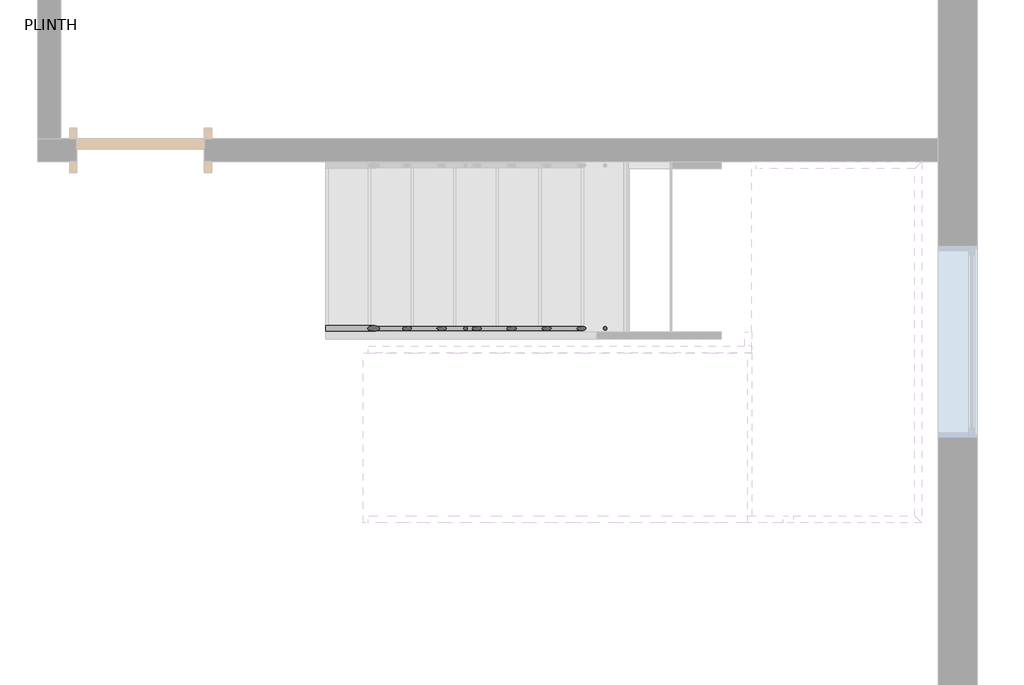
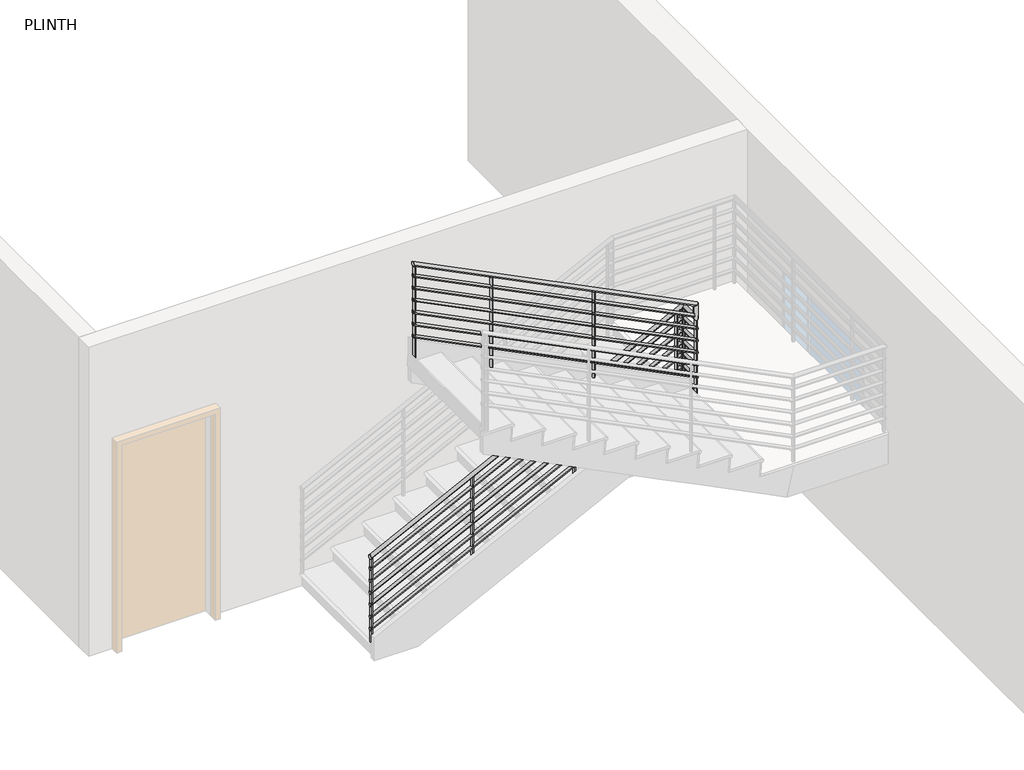
# One storey, part 2 of 4: 1 railing.
"""IFC4 building model written with IfcOpenShell, lengths in millimetres."""

from ifc_helpers import new_model, si_unit, point, frame, frame_2d, origin, place, context, project, spatial, circle_curve, ellipse_curve, trimmed, segment, composite_curve, outline, extrude, element, save
from ifc_brep_helpers import plane_surface, cylinder_surface, advanced_brep

model = new_model("IFC4")

# Units and contexts
model_context = context("Model", 3, world=origin())
ifc_project = project(units=[si_unit("LENGTHUNIT", "METRE", prefix="MILLI")], contexts=[model_context])

# Site, building, storey
site = spatial("IfcSite", under=ifc_project)
building = spatial("IfcBuilding", under=site)
storey = spatial("IfcBuildingStorey", under=building, Name="PLINTH", Elevation=0.0)

# Railing
placement = place(None, origin())
element("IfcRailing", 1, ObjectType="900mm Pipe", at=placement, inside=storey, context=model_context, shape_type="SolidModel", body=[
    advanced_brep(
    [(6849.4583908, 2412.6640673, 1030.0393202), (6849.4583908, 2452.6640673, 1030.0393202), (9913.9141188, 2412.6640673, 2562.2671843), (9949.6912065, 2452.6640673, 2580.1557281)],
    [
        (0, 1, ellipse_curve(frame((6849.4583908, 2432.6640673, 1030.0393202), z_axis=(-1.0, 0.0, 0.0), x_axis=(0.0, 0.0, -1.0)), 22.3606798, 20.0)),
        (1, 0, ellipse_curve(frame((6849.4583908, 2432.6640673, 1030.0393202), z_axis=(-1.0, 0.0, 0.0), x_axis=(0.0, 0.0, -1.0)), 22.3606798, 20.0)),
        (2, 3, ellipse_curve(frame((9931.8026627, 2432.6640673, 2571.2114562), z_axis=(0.632455532033675, -0.7071067811865486, 0.3162277660168374), x_axis=(-0.6324555320336768, -0.7071067811865465, -0.3162277660168383)), 28.2842712, 20.0)),
        (3, 2, ellipse_curve(frame((9931.8026627, 2432.6640673, 2571.2114562), z_axis=(0.632455532033675, -0.7071067811865486, 0.3162277660168374), x_axis=(-0.6324555320336768, -0.7071067811865465, -0.3162277660168383)), 28.2842712, 20.0)),
        (0, 2),
        (3, 1),
    ],
    [
        plane_surface(frame((6849.4583908, 2432.6640673, 1052.4), z_axis=(-1.0, 0.0, 0.0), x_axis=(0.0, 1.0, 0.0))),
        plane_surface(frame((9922.8583908, 2432.6640673, 2589.1), z_axis=(0.6324555320336751, -0.7071067811865487, 0.31622776601683744), x_axis=(0.7745966692414842, 0.5773502691896254, -0.25819888974716015))),
        cylinder_surface(frame((6858.4026627, 2432.6640673, 1034.5114562), z_axis=(-0.894427190999916, 0.0, -0.4472135954999578), x_axis=(0.0, 1.0, 0.0)), 20.0),
    ],
    [
        (0, [[1, 2]]),
        (1, [[3, 4]]),
        (2, [[-1, 5, -4, 6]]),
        (2, [[-2, -6, -3, -5]]),
    ],
),
    advanced_brep(
    [(9902.8583908, 2405.8312516, 2556.4), (9942.8583908, 2441.6083392, 2556.4), (9902.8583908, 2231.8640673, 2556.4), (9942.8583908, 2231.8640673, 2556.4)],
    [
        (0, 1, ellipse_curve(frame((9922.8583908, 2423.7197954, 2556.4), z_axis=(-0.632455532033675, 0.7071067811865486, -0.3162277660168374), x_axis=(0.6324555320336768, 0.7071067811865465, 0.3162277660168383)), 28.2842712, 20.0)),
        (1, 0, ellipse_curve(frame((9922.8583908, 2423.7197954, 2556.4), z_axis=(-0.632455532033675, 0.7071067811865486, -0.3162277660168374), x_axis=(0.6324555320336768, 0.7071067811865465, 0.3162277660168383)), 28.2842712, 20.0)),
        (2, 3, ellipse_curve(frame((9922.8583908, 2231.8640673, 2556.4), z_axis=(0.0, -0.7071067811865476, 0.7071067811865476), x_axis=(0.0, 0.7071067811865474, 0.7071067811865476)), 28.2842712, 20.0)),
        (3, 2, ellipse_curve(frame((9922.8583908, 2231.8640673, 2556.4), z_axis=(0.0, -0.7071067811865476, 0.7071067811865476), x_axis=(0.0, 0.7071067811865474, 0.7071067811865476)), 28.2842712, 20.0)),
        (0, 2),
        (3, 1),
    ],
    [
        plane_surface(frame((9922.8583908, 2432.6640673, 2576.4), z_axis=(-0.6324555320336751, 0.7071067811865487, -0.31622776601683744), x_axis=(0.7745966692414842, 0.5773502691896254, -0.25819888974716015))),
        plane_surface(frame((9922.8583908, 2251.8640673, 2576.4), z_axis=(0.0, -0.7071067811865476, 0.7071067811865476), x_axis=(1.0, 0.0, 0.0))),
        cylinder_surface(frame((9922.8583908, 2432.6640673, 2556.4), z_axis=(0.0, 1.0, 0.0), x_axis=(1.0, 0.0, 0.0)), 20.0),
    ],
    [
        (0, [[1, 2]]),
        (1, [[3, 4]]),
        (2, [[-1, 5, -4, 6]]),
        (2, [[-2, -6, -3, -5]]),
    ],
),
    advanced_brep(
    [(9902.8583908, 2231.8640673, 2556.4), (9942.8583908, 2231.8640673, 2556.4), (9902.8583908, 2231.8640673, 2681.3786405), (9942.8583908, 2231.8640673, 2706.1)],
    [
        (0, 1, ellipse_curve(frame((9922.8583908, 2231.8640673, 2556.4), z_axis=(0.0, 0.7071067811865476, -0.7071067811865476), x_axis=(0.0, -0.7071067811865476, -0.7071067811865474)), 28.2842712, 20.0)),
        (1, 0, ellipse_curve(frame((9922.8583908, 2231.8640673, 2556.4), z_axis=(0.0, 0.7071067811865476, -0.7071067811865476), x_axis=(0.0, -0.7071067811865476, -0.7071067811865474)), 28.2842712, 20.0)),
        (2, 3, ellipse_curve(frame((9922.8583908, 2231.8640673, 2693.7393202), z_axis=(-0.5257311121191335, 0.0, 0.8506508083520401), x_axis=(-0.8506508083520401, 0.0, -0.5257311121191331)), 23.5114101, 20.0)),
        (3, 2, ellipse_curve(frame((9922.8583908, 2231.8640673, 2693.7393202), z_axis=(-0.5257311121191335, 0.0, 0.8506508083520401), x_axis=(-0.8506508083520401, 0.0, -0.5257311121191331)), 23.5114101, 20.0)),
        (0, 2),
        (3, 1),
    ],
    [
        plane_surface(frame((9922.8583908, 2231.8640673, 2556.4), z_axis=(0.0, 0.7071067811865476, -0.7071067811865476), x_axis=(1.0, 0.0, 0.0))),
        plane_surface(frame((9922.8583908, 2231.8640673, 2693.7393202), z_axis=(-0.5257311121191335, 0.0, 0.8506508083520401), x_axis=(0.8506508083520401, 0.0, 0.5257311121191335))),
        cylinder_surface(frame((9922.8583908, 2231.8640673, 2556.4), z_axis=(0.0, 0.0, -1.0), x_axis=(1.0, 0.0, 0.0)), 20.0),
    ],
    [
        (0, [[1, 2]]),
        (1, [[3, 4]]),
        (2, [[-1, 5, -4, 6]]),
        (2, [[-2, -6, -3, -5]]),
    ],
),
    advanced_brep(
    [(9922.8583908, 2251.8640673, 2693.7393202), (9922.8583908, 2211.8640673, 2693.7393202), (7154.2583908, 2251.8640673, 4078.0393202), (7154.2583908, 2211.8640673, 4078.0393202)],
    [
        (0, 1, ellipse_curve(frame((9922.8583908, 2231.8640673, 2693.7393202), z_axis=(0.5257311121191335, 0.0, -0.8506508083520401), x_axis=(0.8506508083520399, 0.0, 0.5257311121191337)), 23.5114101, 20.0)),
        (1, 0, ellipse_curve(frame((9922.8583908, 2231.8640673, 2693.7393202), z_axis=(0.5257311121191335, 0.0, -0.8506508083520401), x_axis=(0.8506508083520399, 0.0, 0.5257311121191337)), 23.5114101, 20.0)),
        (2, 3, ellipse_curve(frame((7154.2583908, 2231.8640673, 4078.0393202), z_axis=(-1.0, 0.0, 0.0), x_axis=(0.0, 0.0, -1.0)), 22.3606798, 20.0)),
        (3, 2, ellipse_curve(frame((7154.2583908, 2231.8640673, 4078.0393202), z_axis=(-1.0, 0.0, 0.0), x_axis=(0.0, 0.0, -1.0)), 22.3606798, 20.0)),
        (0, 2),
        (3, 1),
    ],
    [
        plane_surface(frame((9942.8583908, 2231.8640673, 2706.1), z_axis=(0.5257311121191335, 0.0, -0.8506508083520401), x_axis=(0.8506508083520401, 0.0, 0.5257311121191335))),
        plane_surface(frame((7154.2583908, 2231.8640673, 4100.4), z_axis=(-1.0, 0.0, 0.0), x_axis=(0.0, -1.0, 0.0))),
        cylinder_surface(frame((9933.9141188, 2231.8640673, 2688.2114562), z_axis=(0.8944271909999157, 0.0, -0.44721359549995826), x_axis=(0.0, -1.0, 0.0)), 20.0),
    ],
    [
        (0, [[1, 2]]),
        (1, [[3, 4]]),
        (2, [[-1, 5, -4, 6]]),
        (2, [[-2, -6, -3, -5]]),
    ],
),
    advanced_brep(
    [(6849.4583908, 2447.6640673, 910.6294902), (6849.4583908, 2417.6640673, 910.6294902), (9900.9994104, 2447.6640673, 2436.4), (9900.9994104, 2417.6640673, 2436.4), (9937.8583908, 2447.6640673, 2436.4), (9907.8583908, 2417.6640673, 2436.4), (9937.8583908, 2246.8640673, 2436.4), (9907.8583908, 2246.8640673, 2436.4)],
    [
        (0, 1, ellipse_curve(frame((6849.4583908, 2432.6640673, 910.6294902), z_axis=(-1.0, 0.0, 0.0), x_axis=(0.0, 0.0, -1.0)), 16.7705098, 15.0)),
        (1, 0, ellipse_curve(frame((6849.4583908, 2432.6640673, 910.6294902), z_axis=(-1.0, 0.0, 0.0), x_axis=(0.0, 0.0, -1.0)), 16.7705098, 15.0)),
        (0, 2),
        (2, 3, ellipse_curve(frame((9900.9994104, 2432.6640673, 2436.4), z_axis=(-0.9732489894677302, 0.0, -0.22975292054736124), x_axis=(0.2297529205473615, 0.0, -0.9732489894677302)), 15.4122945, 15.0)),
        (3, 1),
        (3, 2, ellipse_curve(frame((9900.9994104, 2432.6640673, 2436.4), z_axis=(-0.9732489894677302, 0.0, -0.22975292054736124), x_axis=(0.2297529205473615, 0.0, -0.9732489894677302)), 15.4122945, 15.0)),
        (2, 4),
        (4, 5, ellipse_curve(frame((9922.8583908, 2432.6640673, 2436.4), z_axis=(-0.7071067811865465, 0.7071067811865487, 0.0), x_axis=(-0.7071067811865486, -0.7071067811865465, 0.0)), 21.2132034, 15.0)),
        (5, 3),
        (5, 4, ellipse_curve(frame((9922.8583908, 2432.6640673, 2436.4), z_axis=(-0.7071067811865465, 0.7071067811865487, 0.0), x_axis=(-0.7071067811865486, -0.7071067811865465, 0.0)), 21.2132034, 15.0)),
        (6, 7, circle_curve(frame((9922.8583908, 2246.8640673, 2436.4), z_axis=(0.0, -1.0, 0.0), x_axis=(-1.0, 0.0, 0.0)), 15.0)),
        (7, 6, circle_curve(frame((9922.8583908, 2246.8640673, 2436.4), z_axis=(0.0, -1.0, 0.0), x_axis=(-1.0, 0.0, 0.0)), 15.0)),
        (4, 6),
        (7, 5),
    ],
    [
        plane_surface(frame((6849.4583908, 2432.6640673, 927.4), z_axis=(-1.0, 0.0, 0.0), x_axis=(0.0, 1.0, 0.0))),
        cylinder_surface(frame((6856.1665947, 2432.6640673, 913.9835921), z_axis=(-0.8944271909999159, 0.0, -0.447213595499958), x_axis=(0.0, -1.0, 0.0)), 15.0),
        cylinder_surface(frame((9897.4583908, 2432.6640673, 2436.4), z_axis=(-1.0, 0.0, 0.0), x_axis=(0.0, -1.0, 0.0)), 15.0),
        plane_surface(frame((9922.8583908, 2246.8640673, 2451.4), z_axis=(0.0, -1.0, 0.0), x_axis=(0.0, 0.0, -1.0))),
        cylinder_surface(frame((9922.8583908, 2432.6640673, 2436.4), z_axis=(0.0, 1.0, 0.0), x_axis=(-1.0, 0.0, 0.0)), 15.0),
    ],
    [
        (0, [[1, 2]]),
        (1, [[-1, 3, 4, 5]]),
        (1, [[-2, -5, 6, -3]]),
        (2, [[-4, 7, 8, 9]]),
        (2, [[-6, -9, 10, -7]]),
        (3, [[11, 12]]),
        (4, [[-8, 13, -12, 14]]),
        (4, [[-10, -14, -11, -13]]),
    ],
),
    advanced_brep(
    [(9937.8583908, 2216.8640673, 2566.8294902), (9937.8583908, 2246.8640673, 2566.8294902), (7154.2583908, 2216.8640673, 3958.6294902), (7154.2583908, 2246.8640673, 3958.6294902)],
    [
        (0, 1, ellipse_curve(frame((9937.8583908, 2231.8640673, 2566.8294902), z_axis=(1.0, 0.0, 0.0), x_axis=(0.0, 0.0, -1.0)), 16.7705098, 15.0)),
        (1, 0, ellipse_curve(frame((9937.8583908, 2231.8640673, 2566.8294902), z_axis=(1.0, 0.0, 0.0), x_axis=(0.0, 0.0, -1.0)), 16.7705098, 15.0)),
        (2, 3, ellipse_curve(frame((7154.2583908, 2231.8640673, 3958.6294902), z_axis=(-1.0, 0.0, 0.0), x_axis=(0.0, 0.0, -1.0)), 16.7705098, 15.0)),
        (3, 2, ellipse_curve(frame((7154.2583908, 2231.8640673, 3958.6294902), z_axis=(-1.0, 0.0, 0.0), x_axis=(0.0, 0.0, -1.0)), 16.7705098, 15.0)),
        (0, 2),
        (3, 1),
    ],
    [
        plane_surface(frame((9937.8583908, 2231.8640673, 2583.6), z_axis=(1.0, 0.0, 0.0), x_axis=(0.0, -1.0, 0.0))),
        plane_surface(frame((7154.2583908, 2231.8640673, 3975.4), z_axis=(-1.0, 0.0, 0.0), x_axis=(0.0, -1.0, 0.0))),
        cylinder_surface(frame((9931.1501868, 2231.8640673, 2570.1835921), z_axis=(0.8944271909999157, 0.0, -0.44721359549995826), x_axis=(0.0, 1.0, 0.0)), 15.0),
    ],
    [
        (0, [[1, 2]]),
        (1, [[3, 4]]),
        (2, [[-1, 5, -4, 6]]),
        (2, [[-2, -6, -3, -5]]),
    ],
),
    advanced_brep(
    [(6849.4583908, 2447.6640673, 785.6294902), (6849.4583908, 2417.6640673, 785.6294902), (9900.9994104, 2447.6640673, 2311.4), (9900.9994104, 2417.6640673, 2311.4), (9937.8583908, 2447.6640673, 2311.4), (9907.8583908, 2417.6640673, 2311.4), (9937.8583908, 2246.8640673, 2311.4), (9907.8583908, 2246.8640673, 2311.4)],
    [
        (0, 1, ellipse_curve(frame((6849.4583908, 2432.6640673, 785.6294902), z_axis=(-1.0, 0.0, 0.0), x_axis=(0.0, 0.0, -1.0)), 16.7705098, 15.0)),
        (1, 0, ellipse_curve(frame((6849.4583908, 2432.6640673, 785.6294902), z_axis=(-1.0, 0.0, 0.0), x_axis=(0.0, 0.0, -1.0)), 16.7705098, 15.0)),
        (0, 2),
        (2, 3, ellipse_curve(frame((9900.9994104, 2432.6640673, 2311.4), z_axis=(-0.9732489894677303, 0.0, -0.22975292054736124), x_axis=(0.22975292054736246, 0.0, -0.97324898946773)), 15.4122945, 15.0)),
        (3, 1),
        (3, 2, ellipse_curve(frame((9900.9994104, 2432.6640673, 2311.4), z_axis=(-0.9732489894677303, 0.0, -0.22975292054736124), x_axis=(0.22975292054736246, 0.0, -0.97324898946773)), 15.4122945, 15.0)),
        (2, 4),
        (4, 5, ellipse_curve(frame((9922.8583908, 2432.6640673, 2311.4), z_axis=(-0.7071067811865465, 0.7071067811865487, 0.0), x_axis=(-0.7071067811865486, -0.7071067811865465, 0.0)), 21.2132034, 15.0)),
        (5, 3),
        (5, 4, ellipse_curve(frame((9922.8583908, 2432.6640673, 2311.4), z_axis=(-0.7071067811865465, 0.7071067811865487, 0.0), x_axis=(-0.7071067811865486, -0.7071067811865465, 0.0)), 21.2132034, 15.0)),
        (6, 7, circle_curve(frame((9922.8583908, 2246.8640673, 2311.4), z_axis=(0.0, -1.0, 0.0), x_axis=(-1.0, 0.0, 0.0)), 15.0)),
        (7, 6, circle_curve(frame((9922.8583908, 2246.8640673, 2311.4), z_axis=(0.0, -1.0, 0.0), x_axis=(-1.0, 0.0, 0.0)), 15.0)),
        (4, 6),
        (7, 5),
    ],
    [
        plane_surface(frame((6849.4583908, 2432.6640673, 802.4), z_axis=(-1.0, 0.0, 0.0), x_axis=(0.0, 1.0, 0.0))),
        cylinder_surface(frame((6856.1665947, 2432.6640673, 788.9835921), z_axis=(-0.894427190999916, 0.0, -0.447213595499958), x_axis=(0.0, -1.0, 0.0)), 15.0),
        cylinder_surface(frame((9897.4583908, 2432.6640673, 2311.4), z_axis=(-1.0, 0.0, 0.0), x_axis=(0.0, -1.0, 0.0)), 15.0),
        plane_surface(frame((9922.8583908, 2246.8640673, 2326.4), z_axis=(0.0, -1.0, 0.0), x_axis=(0.0, 0.0, -1.0))),
        cylinder_surface(frame((9922.8583908, 2432.6640673, 2311.4), z_axis=(0.0, 1.0, 0.0), x_axis=(-1.0, 0.0, 0.0)), 15.0),
    ],
    [
        (0, [[1, 2]]),
        (1, [[-1, 3, 4, 5]]),
        (1, [[-2, -5, 6, -3]]),
        (2, [[-4, 7, 8, 9]]),
        (2, [[-6, -9, 10, -7]]),
        (3, [[11, 12]]),
        (4, [[-8, 13, -12, 14]]),
        (4, [[-10, -14, -11, -13]]),
    ],
),
    advanced_brep(
    [(9937.8583908, 2216.8640673, 2441.8294902), (9937.8583908, 2246.8640673, 2441.8294902), (7154.2583908, 2216.8640673, 3833.6294902), (7154.2583908, 2246.8640673, 3833.6294902)],
    [
        (0, 1, ellipse_curve(frame((9937.8583908, 2231.8640673, 2441.8294902), z_axis=(1.0, 0.0, 0.0), x_axis=(0.0, 0.0, -1.0)), 16.7705098, 15.0)),
        (1, 0, ellipse_curve(frame((9937.8583908, 2231.8640673, 2441.8294902), z_axis=(1.0, 0.0, 0.0), x_axis=(0.0, 0.0, -1.0)), 16.7705098, 15.0)),
        (2, 3, ellipse_curve(frame((7154.2583908, 2231.8640673, 3833.6294902), z_axis=(-1.0, 0.0, 0.0), x_axis=(0.0, 0.0, -1.0)), 16.7705098, 15.0)),
        (3, 2, ellipse_curve(frame((7154.2583908, 2231.8640673, 3833.6294902), z_axis=(-1.0, 0.0, 0.0), x_axis=(0.0, 0.0, -1.0)), 16.7705098, 15.0)),
        (0, 2),
        (3, 1),
    ],
    [
        plane_surface(frame((9937.8583908, 2231.8640673, 2458.6), z_axis=(1.0, 0.0, 0.0), x_axis=(0.0, -1.0, 0.0))),
        plane_surface(frame((7154.2583908, 2231.8640673, 3850.4), z_axis=(-1.0, 0.0, 0.0), x_axis=(0.0, -1.0, 0.0))),
        cylinder_surface(frame((9931.1501868, 2231.8640673, 2445.1835921), z_axis=(0.8944271909999157, 0.0, -0.44721359549995826), x_axis=(0.0, 1.0, 0.0)), 15.0),
    ],
    [
        (0, [[1, 2]]),
        (1, [[3, 4]]),
        (2, [[-1, 5, -4, 6]]),
        (2, [[-2, -6, -3, -5]]),
    ],
),
    advanced_brep(
    [(6849.4583908, 2447.6640673, 660.6294902), (6849.4583908, 2417.6640673, 660.6294902), (9900.9994104, 2447.6640673, 2186.4), (9900.9994104, 2417.6640673, 2186.4), (9937.8583908, 2447.6640673, 2186.4), (9907.8583908, 2417.6640673, 2186.4), (9937.8583908, 2246.8640673, 2186.4), (9907.8583908, 2246.8640673, 2186.4)],
    [
        (0, 1, ellipse_curve(frame((6849.4583908, 2432.6640673, 660.6294902), z_axis=(-1.0, 0.0, 0.0), x_axis=(0.0, 0.0, -1.0)), 16.7705098, 15.0)),
        (1, 0, ellipse_curve(frame((6849.4583908, 2432.6640673, 660.6294902), z_axis=(-1.0, 0.0, 0.0), x_axis=(0.0, 0.0, -1.0)), 16.7705098, 15.0)),
        (0, 2),
        (2, 3, ellipse_curve(frame((9900.9994104, 2432.6640673, 2186.4), z_axis=(-0.9732489894677303, 0.0, -0.22975292054736124), x_axis=(0.22975292054736246, 0.0, -0.97324898946773)), 15.4122945, 15.0)),
        (3, 1),
        (3, 2, ellipse_curve(frame((9900.9994104, 2432.6640673, 2186.4), z_axis=(-0.9732489894677303, 0.0, -0.22975292054736124), x_axis=(0.22975292054736246, 0.0, -0.97324898946773)), 15.4122945, 15.0)),
        (2, 4),
        (4, 5, ellipse_curve(frame((9922.8583908, 2432.6640673, 2186.4), z_axis=(-0.7071067811865465, 0.7071067811865487, 0.0), x_axis=(-0.7071067811865486, -0.7071067811865465, 0.0)), 21.2132034, 15.0)),
        (5, 3),
        (5, 4, ellipse_curve(frame((9922.8583908, 2432.6640673, 2186.4), z_axis=(-0.7071067811865465, 0.7071067811865487, 0.0), x_axis=(-0.7071067811865486, -0.7071067811865465, 0.0)), 21.2132034, 15.0)),
        (6, 7, circle_curve(frame((9922.8583908, 2246.8640673, 2186.4), z_axis=(0.0, -1.0, 0.0), x_axis=(-1.0, 0.0, 0.0)), 15.0)),
        (7, 6, circle_curve(frame((9922.8583908, 2246.8640673, 2186.4), z_axis=(0.0, -1.0, 0.0), x_axis=(-1.0, 0.0, 0.0)), 15.0)),
        (4, 6),
        (7, 5),
    ],
    [
        plane_surface(frame((6849.4583908, 2432.6640673, 677.4), z_axis=(-1.0, 0.0, 0.0), x_axis=(0.0, 1.0, 0.0))),
        cylinder_surface(frame((6856.1665947, 2432.6640673, 663.9835921), z_axis=(-0.894427190999916, 0.0, -0.447213595499958), x_axis=(0.0, -1.0, 0.0)), 15.0),
        cylinder_surface(frame((9897.4583908, 2432.6640673, 2186.4), z_axis=(-1.0, 0.0, 0.0), x_axis=(0.0, -1.0, 0.0)), 15.0),
        plane_surface(frame((9922.8583908, 2246.8640673, 2201.4), z_axis=(0.0, -1.0, 0.0), x_axis=(0.0, 0.0, -1.0))),
        cylinder_surface(frame((9922.8583908, 2432.6640673, 2186.4), z_axis=(0.0, 1.0, 0.0), x_axis=(-1.0, 0.0, 0.0)), 15.0),
    ],
    [
        (0, [[1, 2]]),
        (1, [[-1, 3, 4, 5]]),
        (1, [[-2, -5, 6, -3]]),
        (2, [[-4, 7, 8, 9]]),
        (2, [[-6, -9, 10, -7]]),
        (3, [[11, 12]]),
        (4, [[-8, 13, -12, 14]]),
        (4, [[-10, -14, -11, -13]]),
    ],
),
    advanced_brep(
    [(9937.8583908, 2216.8640673, 2316.8294902), (9937.8583908, 2246.8640673, 2316.8294902), (7154.2583908, 2216.8640673, 3708.6294902), (7154.2583908, 2246.8640673, 3708.6294902)],
    [
        (0, 1, ellipse_curve(frame((9937.8583908, 2231.8640673, 2316.8294902), z_axis=(1.0, 0.0, 0.0), x_axis=(0.0, 0.0, -1.0)), 16.7705098, 15.0)),
        (1, 0, ellipse_curve(frame((9937.8583908, 2231.8640673, 2316.8294902), z_axis=(1.0, 0.0, 0.0), x_axis=(0.0, 0.0, -1.0)), 16.7705098, 15.0)),
        (2, 3, ellipse_curve(frame((7154.2583908, 2231.8640673, 3708.6294902), z_axis=(-1.0, 0.0, 0.0), x_axis=(0.0, 0.0, -1.0)), 16.7705098, 15.0)),
        (3, 2, ellipse_curve(frame((7154.2583908, 2231.8640673, 3708.6294902), z_axis=(-1.0, 0.0, 0.0), x_axis=(0.0, 0.0, -1.0)), 16.7705098, 15.0)),
        (0, 2),
        (3, 1),
    ],
    [
        plane_surface(frame((9937.8583908, 2231.8640673, 2333.6), z_axis=(1.0, 0.0, 0.0), x_axis=(0.0, -1.0, 0.0))),
        plane_surface(frame((7154.2583908, 2231.8640673, 3725.4), z_axis=(-1.0, 0.0, 0.0), x_axis=(0.0, -1.0, 0.0))),
        cylinder_surface(frame((9931.1501868, 2231.8640673, 2320.1835921), z_axis=(0.8944271909999157, 0.0, -0.4472135954999583), x_axis=(0.0, 1.0, 0.0)), 15.0),
    ],
    [
        (0, [[1, 2]]),
        (1, [[3, 4]]),
        (2, [[-1, 5, -4, 6]]),
        (2, [[-2, -6, -3, -5]]),
    ],
),
    advanced_brep(
    [(6849.4583908, 2447.6640673, 535.6294902), (6849.4583908, 2417.6640673, 535.6294902), (9900.9994104, 2447.6640673, 2061.4), (9900.9994104, 2417.6640673, 2061.4), (9937.8583908, 2447.6640673, 2061.4), (9907.8583908, 2417.6640673, 2061.4), (9937.8583908, 2246.8640673, 2061.4), (9907.8583908, 2246.8640673, 2061.4)],
    [
        (0, 1, ellipse_curve(frame((6849.4583908, 2432.6640673, 535.6294902), z_axis=(-1.0, 0.0, 0.0), x_axis=(0.0, 0.0, -1.0)), 16.7705098, 15.0)),
        (1, 0, ellipse_curve(frame((6849.4583908, 2432.6640673, 535.6294902), z_axis=(-1.0, 0.0, 0.0), x_axis=(0.0, 0.0, -1.0)), 16.7705098, 15.0)),
        (0, 2),
        (2, 3, ellipse_curve(frame((9900.9994104, 2432.6640673, 2061.4), z_axis=(-0.9732489894677303, 0.0, -0.22975292054736124), x_axis=(0.22975292054736246, 0.0, -0.97324898946773)), 15.4122945, 15.0)),
        (3, 1),
        (3, 2, ellipse_curve(frame((9900.9994104, 2432.6640673, 2061.4), z_axis=(-0.9732489894677303, 0.0, -0.22975292054736124), x_axis=(0.22975292054736246, 0.0, -0.97324898946773)), 15.4122945, 15.0)),
        (2, 4),
        (4, 5, ellipse_curve(frame((9922.8583908, 2432.6640673, 2061.4), z_axis=(-0.7071067811865465, 0.7071067811865487, 0.0), x_axis=(-0.7071067811865486, -0.7071067811865465, 0.0)), 21.2132034, 15.0)),
        (5, 3),
        (5, 4, ellipse_curve(frame((9922.8583908, 2432.6640673, 2061.4), z_axis=(-0.7071067811865465, 0.7071067811865487, 0.0), x_axis=(-0.7071067811865486, -0.7071067811865465, 0.0)), 21.2132034, 15.0)),
        (6, 7, circle_curve(frame((9922.8583908, 2246.8640673, 2061.4), z_axis=(0.0, -1.0, 0.0), x_axis=(-1.0, 0.0, 0.0)), 15.0)),
        (7, 6, circle_curve(frame((9922.8583908, 2246.8640673, 2061.4), z_axis=(0.0, -1.0, 0.0), x_axis=(-1.0, 0.0, 0.0)), 15.0)),
        (4, 6),
        (7, 5),
    ],
    [
        plane_surface(frame((6849.4583908, 2432.6640673, 552.4), z_axis=(-1.0, 0.0, 0.0), x_axis=(0.0, 1.0, 0.0))),
        cylinder_surface(frame((6856.1665947, 2432.6640673, 538.9835921), z_axis=(-0.894427190999916, 0.0, -0.447213595499958), x_axis=(0.0, -1.0, 0.0)), 15.0),
        cylinder_surface(frame((9897.4583908, 2432.6640673, 2061.4), z_axis=(-1.0, 0.0, 0.0), x_axis=(0.0, -1.0, 0.0)), 15.0),
        plane_surface(frame((9922.8583908, 2246.8640673, 2076.4), z_axis=(0.0, -1.0, 0.0), x_axis=(0.0, 0.0, -1.0))),
        cylinder_surface(frame((9922.8583908, 2432.6640673, 2061.4), z_axis=(0.0, 1.0, 0.0), x_axis=(-1.0, 0.0, 0.0)), 15.0),
    ],
    [
        (0, [[1, 2]]),
        (1, [[-1, 3, 4, 5]]),
        (1, [[-2, -5, 6, -3]]),
        (2, [[-4, 7, 8, 9]]),
        (2, [[-6, -9, 10, -7]]),
        (3, [[11, 12]]),
        (4, [[-8, 13, -12, 14]]),
        (4, [[-10, -14, -11, -13]]),
    ],
),
    advanced_brep(
    [(9937.8583908, 2216.8640673, 2191.8294902), (9937.8583908, 2246.8640673, 2191.8294902), (7154.2583908, 2216.8640673, 3583.6294902), (7154.2583908, 2246.8640673, 3583.6294902)],
    [
        (0, 1, ellipse_curve(frame((9937.8583908, 2231.8640673, 2191.8294902), z_axis=(1.0, 0.0, 0.0), x_axis=(0.0, 0.0, -1.0)), 16.7705098, 15.0)),
        (1, 0, ellipse_curve(frame((9937.8583908, 2231.8640673, 2191.8294902), z_axis=(1.0, 0.0, 0.0), x_axis=(0.0, 0.0, -1.0)), 16.7705098, 15.0)),
        (2, 3, ellipse_curve(frame((7154.2583908, 2231.8640673, 3583.6294902), z_axis=(-1.0, 0.0, 0.0), x_axis=(0.0, 0.0, -1.0)), 16.7705098, 15.0)),
        (3, 2, ellipse_curve(frame((7154.2583908, 2231.8640673, 3583.6294902), z_axis=(-1.0, 0.0, 0.0), x_axis=(0.0, 0.0, -1.0)), 16.7705098, 15.0)),
        (0, 2),
        (3, 1),
    ],
    [
        plane_surface(frame((9937.8583908, 2231.8640673, 2208.6), z_axis=(1.0, 0.0, 0.0), x_axis=(0.0, -1.0, 0.0))),
        plane_surface(frame((7154.2583908, 2231.8640673, 3600.4), z_axis=(-1.0, 0.0, 0.0), x_axis=(0.0, -1.0, 0.0))),
        cylinder_surface(frame((9931.1501868, 2231.8640673, 2195.1835921), z_axis=(0.8944271909999157, 0.0, -0.44721359549995826), x_axis=(0.0, 1.0, 0.0)), 15.0),
    ],
    [
        (0, [[1, 2]]),
        (1, [[3, 4]]),
        (2, [[-1, 5, -4, 6]]),
        (2, [[-2, -6, -3, -5]]),
    ],
),
    advanced_brep(
    [(6849.4583908, 2447.6640673, 410.6294902), (6849.4583908, 2417.6640673, 410.6294902), (9900.9994104, 2447.6640673, 1936.4), (9900.9994104, 2417.6640673, 1936.4), (9937.8583908, 2447.6640673, 1936.4), (9907.8583908, 2417.6640673, 1936.4), (9937.8583908, 2246.8640673, 1936.4), (9907.8583908, 2246.8640673, 1936.4)],
    [
        (0, 1, ellipse_curve(frame((6849.4583908, 2432.6640673, 410.6294902), z_axis=(-1.0, 0.0, 0.0), x_axis=(0.0, 0.0, -1.0)), 16.7705098, 15.0)),
        (1, 0, ellipse_curve(frame((6849.4583908, 2432.6640673, 410.6294902), z_axis=(-1.0, 0.0, 0.0), x_axis=(0.0, 0.0, -1.0)), 16.7705098, 15.0)),
        (0, 2),
        (2, 3, ellipse_curve(frame((9900.9994104, 2432.6640673, 1936.4), z_axis=(-0.9732489894677303, 0.0, -0.22975292054736124), x_axis=(0.22975292054736246, 0.0, -0.97324898946773)), 15.4122945, 15.0)),
        (3, 1),
        (3, 2, ellipse_curve(frame((9900.9994104, 2432.6640673, 1936.4), z_axis=(-0.9732489894677303, 0.0, -0.22975292054736124), x_axis=(0.22975292054736246, 0.0, -0.97324898946773)), 15.4122945, 15.0)),
        (2, 4),
        (4, 5, ellipse_curve(frame((9922.8583908, 2432.6640673, 1936.4), z_axis=(-0.7071067811865465, 0.7071067811865487, 0.0), x_axis=(-0.7071067811865486, -0.7071067811865465, 0.0)), 21.2132034, 15.0)),
        (5, 3),
        (5, 4, ellipse_curve(frame((9922.8583908, 2432.6640673, 1936.4), z_axis=(-0.7071067811865465, 0.7071067811865487, 0.0), x_axis=(-0.7071067811865486, -0.7071067811865465, 0.0)), 21.2132034, 15.0)),
        (6, 7, circle_curve(frame((9922.8583908, 2246.8640673, 1936.4), z_axis=(0.0, -1.0, 0.0), x_axis=(-1.0, 0.0, 0.0)), 15.0)),
        (7, 6, circle_curve(frame((9922.8583908, 2246.8640673, 1936.4), z_axis=(0.0, -1.0, 0.0), x_axis=(-1.0, 0.0, 0.0)), 15.0)),
        (4, 6),
        (7, 5),
    ],
    [
        plane_surface(frame((6849.4583908, 2432.6640673, 427.4), z_axis=(-1.0, 0.0, 0.0), x_axis=(0.0, 1.0, 0.0))),
        cylinder_surface(frame((6856.1665947, 2432.6640673, 413.9835921), z_axis=(-0.894427190999916, 0.0, -0.447213595499958), x_axis=(0.0, -1.0, 0.0)), 15.0),
        cylinder_surface(frame((9897.4583908, 2432.6640673, 1936.4), z_axis=(-1.0, 0.0, 0.0), x_axis=(0.0, -1.0, 0.0)), 15.0),
        plane_surface(frame((9922.8583908, 2246.8640673, 1951.4), z_axis=(0.0, -1.0, 0.0), x_axis=(0.0, 0.0, -1.0))),
        cylinder_surface(frame((9922.8583908, 2432.6640673, 1936.4), z_axis=(0.0, 1.0, 0.0), x_axis=(-1.0, 0.0, 0.0)), 15.0),
    ],
    [
        (0, [[1, 2]]),
        (1, [[-1, 3, 4, 5]]),
        (1, [[-2, -5, 6, -3]]),
        (2, [[-4, 7, 8, 9]]),
        (2, [[-6, -9, 10, -7]]),
        (3, [[11, 12]]),
        (4, [[-8, 13, -12, 14]]),
        (4, [[-10, -14, -11, -13]]),
    ],
),
    advanced_brep(
    [(9937.8583908, 2216.8640673, 2066.8294902), (9937.8583908, 2246.8640673, 2066.8294902), (7154.2583908, 2216.8640673, 3458.6294902), (7154.2583908, 2246.8640673, 3458.6294902)],
    [
        (0, 1, ellipse_curve(frame((9937.8583908, 2231.8640673, 2066.8294902), z_axis=(1.0, 0.0, 0.0), x_axis=(0.0, 0.0, -0.9999999999999999)), 16.7705098, 15.0)),
        (1, 0, ellipse_curve(frame((9937.8583908, 2231.8640673, 2066.8294902), z_axis=(1.0, 0.0, 0.0), x_axis=(0.0, 0.0, -0.9999999999999999)), 16.7705098, 15.0)),
        (2, 3, ellipse_curve(frame((7154.2583908, 2231.8640673, 3458.6294902), z_axis=(-1.0, 0.0, 0.0), x_axis=(0.0, 0.0, -0.9999999999999999)), 16.7705098, 15.0)),
        (3, 2, ellipse_curve(frame((7154.2583908, 2231.8640673, 3458.6294902), z_axis=(-1.0, 0.0, 0.0), x_axis=(0.0, 0.0, -0.9999999999999999)), 16.7705098, 15.0)),
        (0, 2),
        (3, 1),
    ],
    [
        plane_surface(frame((9937.8583908, 2231.8640673, 2083.6), z_axis=(1.0, 0.0, 0.0), x_axis=(0.0, -1.0, 0.0))),
        plane_surface(frame((7154.2583908, 2231.8640673, 3475.4), z_axis=(-1.0, 0.0, 0.0), x_axis=(0.0, -1.0, 0.0))),
        cylinder_surface(frame((9931.1501868, 2231.8640673, 2070.1835921), z_axis=(0.8944271909999159, 0.0, -0.44721359549995815), x_axis=(0.0, 1.0, 0.0)), 15.0),
    ],
    [
        (0, [[1, 2]]),
        (1, [[3, 4]]),
        (2, [[-1, 5, -4, 6]]),
        (2, [[-2, -6, -3, -5]]),
    ],
),
    advanced_brep(
    [(6849.4583908, 2447.6640673, 285.6294902), (6849.4583908, 2417.6640673, 285.6294902), (9900.9994104, 2447.6640673, 1811.4), (9900.9994104, 2417.6640673, 1811.4), (9937.8583908, 2447.6640673, 1811.4), (9907.8583908, 2417.6640673, 1811.4), (9937.8583908, 2246.8640673, 1811.4), (9907.8583908, 2246.8640673, 1811.4)],
    [
        (0, 1, ellipse_curve(frame((6849.4583908, 2432.6640673, 285.6294902), z_axis=(-1.0, 0.0, 0.0), x_axis=(0.0, 0.0, -1.0)), 16.7705098, 15.0)),
        (1, 0, ellipse_curve(frame((6849.4583908, 2432.6640673, 285.6294902), z_axis=(-1.0, 0.0, 0.0), x_axis=(0.0, 0.0, -1.0)), 16.7705098, 15.0)),
        (0, 2),
        (2, 3, ellipse_curve(frame((9900.9994104, 2432.6640673, 1811.4), z_axis=(-0.9732489894677303, 0.0, -0.22975292054736124), x_axis=(0.22975292054736246, 0.0, -0.97324898946773)), 15.4122945, 15.0)),
        (3, 1),
        (3, 2, ellipse_curve(frame((9900.9994104, 2432.6640673, 1811.4), z_axis=(-0.9732489894677303, 0.0, -0.22975292054736124), x_axis=(0.22975292054736246, 0.0, -0.97324898946773)), 15.4122945, 15.0)),
        (2, 4),
        (4, 5, ellipse_curve(frame((9922.8583908, 2432.6640673, 1811.4), z_axis=(-0.7071067811865465, 0.7071067811865487, 0.0), x_axis=(-0.7071067811865486, -0.7071067811865465, 0.0)), 21.2132034, 15.0)),
        (5, 3),
        (5, 4, ellipse_curve(frame((9922.8583908, 2432.6640673, 1811.4), z_axis=(-0.7071067811865465, 0.7071067811865487, 0.0), x_axis=(-0.7071067811865486, -0.7071067811865465, 0.0)), 21.2132034, 15.0)),
        (6, 7, circle_curve(frame((9922.8583908, 2246.8640673, 1811.4), z_axis=(0.0, -1.0, 0.0), x_axis=(-1.0, 0.0, 0.0)), 15.0)),
        (7, 6, circle_curve(frame((9922.8583908, 2246.8640673, 1811.4), z_axis=(0.0, -1.0, 0.0), x_axis=(-1.0, 0.0, 0.0)), 15.0)),
        (4, 6),
        (7, 5),
    ],
    [
        plane_surface(frame((6849.4583908, 2432.6640673, 302.4), z_axis=(-1.0, 0.0, 0.0), x_axis=(0.0, 1.0, 0.0))),
        cylinder_surface(frame((6856.1665947, 2432.6640673, 288.9835921), z_axis=(-0.894427190999916, 0.0, -0.447213595499958), x_axis=(0.0, -1.0, 0.0)), 15.0),
        cylinder_surface(frame((9897.4583908, 2432.6640673, 1811.4), z_axis=(-1.0, 0.0, 0.0), x_axis=(0.0, -1.0, 0.0)), 15.0),
        plane_surface(frame((9922.8583908, 2246.8640673, 1826.4), z_axis=(0.0, -1.0, 0.0), x_axis=(0.0, 0.0, -1.0))),
        cylinder_surface(frame((9922.8583908, 2432.6640673, 1811.4), z_axis=(0.0, 1.0, 0.0), x_axis=(-1.0, 0.0, 0.0)), 15.0),
    ],
    [
        (0, [[1, 2]]),
        (1, [[-1, 3, 4, 5]]),
        (1, [[-2, -5, 6, -3]]),
        (2, [[-4, 7, 8, 9]]),
        (2, [[-6, -9, 10, -7]]),
        (3, [[11, 12]]),
        (4, [[-8, 13, -12, 14]]),
        (4, [[-10, -14, -11, -13]]),
    ],
),
    advanced_brep(
    [(9937.8583908, 2216.8640673, 1941.8294902), (9937.8583908, 2246.8640673, 1941.8294902), (7154.2583908, 2216.8640673, 3333.6294902), (7154.2583908, 2246.8640673, 3333.6294902)],
    [
        (0, 1, ellipse_curve(frame((9937.8583908, 2231.8640673, 1941.8294902), z_axis=(1.0, 0.0, 0.0), x_axis=(0.0, 0.0, -1.0)), 16.7705098, 15.0)),
        (1, 0, ellipse_curve(frame((9937.8583908, 2231.8640673, 1941.8294902), z_axis=(1.0, 0.0, 0.0), x_axis=(0.0, 0.0, -1.0)), 16.7705098, 15.0)),
        (2, 3, ellipse_curve(frame((7154.2583908, 2231.8640673, 3333.6294902), z_axis=(-1.0, 0.0, 0.0), x_axis=(0.0, 0.0, -1.0)), 16.7705098, 15.0)),
        (3, 2, ellipse_curve(frame((7154.2583908, 2231.8640673, 3333.6294902), z_axis=(-1.0, 0.0, 0.0), x_axis=(0.0, 0.0, -1.0)), 16.7705098, 15.0)),
        (0, 2),
        (3, 1),
    ],
    [
        plane_surface(frame((9937.8583908, 2231.8640673, 1958.6), z_axis=(1.0, 0.0, 0.0), x_axis=(0.0, -1.0, 0.0))),
        plane_surface(frame((7154.2583908, 2231.8640673, 3350.4), z_axis=(-1.0, 0.0, 0.0), x_axis=(0.0, -1.0, 0.0))),
        cylinder_surface(frame((9931.1501868, 2231.8640673, 1945.1835921), z_axis=(0.8944271909999157, 0.0, -0.44721359549995826), x_axis=(0.0, 1.0, 0.0)), 15.0),
    ],
    [
        (0, [[1, 2]]),
        (1, [[3, 4]]),
        (2, [[-1, 5, -4, 6]]),
        (2, [[-2, -6, -3, -5]]),
    ],
),
    advanced_brep(
    [(7922.8583908, 2244.3640673, 3671.3786405), (7922.8583908, 2244.3640673, 2743.2), (7922.8583908, 2219.3640673, 2743.2), (7922.8583908, 2219.3640673, 3671.3786405)],
    [
        (0, 1),
        (1, 2, circle_curve(frame((7922.8583908, 2231.8640673, 2743.2), z_axis=(0.0, 0.0, 1.0), x_axis=(0.0, -1.0, 0.0)), 12.5)),
        (2, 3),
        (3, 0, ellipse_curve(frame((7922.8583908, 2231.8640673, 3671.3786405), z_axis=(-0.447213595499958, 0.0, -0.894427190999916), x_axis=(-0.8944271909999161, 0.0, 0.4472135954999576)), 13.9754249, 12.5)),
        (0, 3, ellipse_curve(frame((7922.8583908, 2231.8640673, 3671.3786405), z_axis=(-0.447213595499958, 0.0, -0.894427190999916), x_axis=(-0.8944271909999161, 0.0, 0.4472135954999576)), 13.9754249, 12.5)),
        (2, 1, circle_curve(frame((7922.8583908, 2231.8640673, 2743.2), z_axis=(0.0, 0.0, 1.0), x_axis=(0.0, -1.0, 0.0)), 12.5)),
    ],
    [
        cylinder_surface(frame((7922.8583908, 2231.8640673, 2643.2), z_axis=(0.0, 0.0, 1.0), x_axis=(0.0, -1.0, 0.0)), 12.5),
        plane_surface(frame((7897.8583908, 2206.8640673, 3683.8786405), z_axis=(0.447213595499958, 0.0, 0.894427190999916), x_axis=(0.0, 1.0, 0.0))),
        plane_surface(frame((7947.8583908, 2206.8640673, 2743.2), z_axis=(0.0, 0.0, -1.0), x_axis=(0.0, 1.0, 0.0))),
    ],
    [
        (0, [[1, 2, 3, 4]]),
        (0, [[-1, 5, -3, 6]]),
        (1, [[-4, -5]]),
        (2, [[-2, -6]]),
    ],
),
    advanced_brep(
    [(8922.8583908, 2244.3640673, 3171.3786405), (8922.8583908, 2244.3640673, 2286.0), (8922.8583908, 2219.3640673, 2286.0), (8922.8583908, 2219.3640673, 3171.3786405)],
    [
        (0, 1),
        (1, 2, circle_curve(frame((8922.8583908, 2231.8640673, 2286.0), z_axis=(0.0, 0.0, 1.0), x_axis=(0.0, -1.0, 0.0)), 12.5)),
        (2, 3),
        (3, 0, ellipse_curve(frame((8922.8583908, 2231.8640673, 3171.3786405), z_axis=(-0.447213595499958, 0.0, -0.894427190999916), x_axis=(-0.8944271909999161, 0.0, 0.4472135954999576)), 13.9754249, 12.5)),
        (0, 3, ellipse_curve(frame((8922.8583908, 2231.8640673, 3171.3786405), z_axis=(-0.447213595499958, 0.0, -0.894427190999916), x_axis=(-0.8944271909999161, 0.0, 0.4472135954999576)), 13.9754249, 12.5)),
        (2, 1, circle_curve(frame((8922.8583908, 2231.8640673, 2286.0), z_axis=(0.0, 0.0, 1.0), x_axis=(0.0, -1.0, 0.0)), 12.5)),
    ],
    [
        cylinder_surface(frame((8922.8583908, 2231.8640673, 2186.0), z_axis=(0.0, 0.0, 1.0), x_axis=(0.0, -1.0, 0.0)), 12.5),
        plane_surface(frame((8897.8583908, 2206.8640673, 3183.8786405), z_axis=(0.447213595499958, 0.0, 0.894427190999916), x_axis=(0.0, 1.0, 0.0))),
        plane_surface(frame((8947.8583908, 2206.8640673, 2286.0), z_axis=(0.0, 0.0, -1.0), x_axis=(0.0, 1.0, 0.0))),
    ],
    [
        (0, [[1, 2, 3, 4]]),
        (0, [[-1, 5, -3, 6]]),
        (1, [[-4, -5]]),
        (2, [[-2, -6]]),
    ],
),
    advanced_brep(
    [(9849.4583908, 2420.1640673, 2507.6786405), (9849.4583908, 2420.1640673, 1524.0), (9849.4583908, 2445.1640673, 1524.0), (9849.4583908, 2445.1640673, 2507.6786405)],
    [
        (0, 1),
        (1, 2, circle_curve(frame((9849.4583908, 2432.6640673, 1524.0), z_axis=(0.0, 0.0, 1.0), x_axis=(0.0, 1.0, 0.0)), 12.5)),
        (2, 3),
        (3, 0, ellipse_curve(frame((9849.4583908, 2432.6640673, 2507.6786405), z_axis=(0.447213595499958, 0.0, -0.894427190999916), x_axis=(0.8944271909999161, 0.0, 0.4472135954999576)), 13.9754249, 12.5)),
        (0, 3, ellipse_curve(frame((9849.4583908, 2432.6640673, 2507.6786405), z_axis=(0.447213595499958, 0.0, -0.894427190999916), x_axis=(0.8944271909999161, 0.0, 0.4472135954999576)), 13.9754249, 12.5)),
        (2, 1, circle_curve(frame((9849.4583908, 2432.6640673, 1524.0), z_axis=(0.0, 0.0, 1.0), x_axis=(0.0, 1.0, 0.0)), 12.5)),
    ],
    [
        cylinder_surface(frame((9849.4583908, 2432.6640673, 1424.0), z_axis=(0.0, 0.0, 1.0), x_axis=(0.0, 1.0, 0.0)), 12.5),
        plane_surface(frame((9874.4583908, 2457.6640673, 2520.1786405), z_axis=(-0.447213595499958, 0.0, 0.894427190999916), x_axis=(0.0, -1.0, 0.0))),
        plane_surface(frame((9824.4583908, 2457.6640673, 1524.0), z_axis=(0.0, 0.0, -1.0), x_axis=(0.0, -1.0, 0.0))),
    ],
    [
        (0, [[1, 2, 3, 4]]),
        (0, [[-1, 5, -3, 6]]),
        (1, [[-4, -5]]),
        (2, [[-2, -6]]),
    ],
),
    advanced_brep(
    [(8849.4583908, 2420.1640673, 2007.6786405), (8849.4583908, 2420.1640673, 1066.8), (8849.4583908, 2445.1640673, 1066.8), (8849.4583908, 2445.1640673, 2007.6786405)],
    [
        (0, 1),
        (1, 2, circle_curve(frame((8849.4583908, 2432.6640673, 1066.8), z_axis=(0.0, 0.0, 1.0), x_axis=(0.0, 1.0, 0.0)), 12.5)),
        (2, 3),
        (3, 0, ellipse_curve(frame((8849.4583908, 2432.6640673, 2007.6786405), z_axis=(0.447213595499958, 0.0, -0.894427190999916), x_axis=(0.8944271909999161, 0.0, 0.4472135954999576)), 13.9754249, 12.5)),
        (0, 3, ellipse_curve(frame((8849.4583908, 2432.6640673, 2007.6786405), z_axis=(0.447213595499958, 0.0, -0.894427190999916), x_axis=(0.8944271909999161, 0.0, 0.4472135954999576)), 13.9754249, 12.5)),
        (2, 1, circle_curve(frame((8849.4583908, 2432.6640673, 1066.8), z_axis=(0.0, 0.0, 1.0), x_axis=(0.0, 1.0, 0.0)), 12.5)),
    ],
    [
        cylinder_surface(frame((8849.4583908, 2432.6640673, 966.8), z_axis=(0.0, 0.0, 1.0), x_axis=(0.0, 1.0, 0.0)), 12.5),
        plane_surface(frame((8874.4583908, 2457.6640673, 2020.1786405), z_axis=(-0.447213595499958, 0.0, 0.894427190999916), x_axis=(0.0, -1.0, 0.0))),
        plane_surface(frame((8824.4583908, 2457.6640673, 1066.8), z_axis=(0.0, 0.0, -1.0), x_axis=(0.0, -1.0, 0.0))),
    ],
    [
        (0, [[1, 2, 3, 4]]),
        (0, [[-1, 5, -3, 6]]),
        (1, [[-4, -5]]),
        (2, [[-2, -6]]),
    ],
),
    advanced_brep(
    [(7849.4583908, 2420.1640673, 1507.6786405), (7849.4583908, 2420.1640673, 609.6), (7849.4583908, 2445.1640673, 609.6), (7849.4583908, 2445.1640673, 1507.6786405)],
    [
        (0, 1),
        (1, 2, circle_curve(frame((7849.4583908, 2432.6640673, 609.6), z_axis=(0.0, 0.0, 1.0), x_axis=(0.0, 1.0, 0.0)), 12.5)),
        (2, 3),
        (3, 0, ellipse_curve(frame((7849.4583908, 2432.6640673, 1507.6786405), z_axis=(0.44721359549995604, 0.0, -0.894427190999917), x_axis=(0.8944271909999172, 0.0, 0.4472135954999556)), 13.9754249, 12.5)),
        (0, 3, ellipse_curve(frame((7849.4583908, 2432.6640673, 1507.6786405), z_axis=(0.44721359549995604, 0.0, -0.894427190999917), x_axis=(0.8944271909999172, 0.0, 0.4472135954999556)), 13.9754249, 12.5)),
        (2, 1, circle_curve(frame((7849.4583908, 2432.6640673, 609.6), z_axis=(0.0, 0.0, 1.0), x_axis=(0.0, 1.0, 0.0)), 12.5)),
    ],
    [
        cylinder_surface(frame((7849.4583908, 2432.6640673, 509.6), z_axis=(0.0, 0.0, 1.0), x_axis=(0.0, 1.0, 0.0)), 12.5),
        plane_surface(frame((7874.4583908, 2457.6640673, 1520.1786405), z_axis=(-0.44721359549995604, 0.0, 0.894427190999917), x_axis=(0.0, -1.0, 0.0))),
        plane_surface(frame((7824.4583908, 2457.6640673, 609.6), z_axis=(0.0, 0.0, -1.0), x_axis=(0.0, -1.0, 0.0))),
    ],
    [
        (0, [[1, 2, 3, 4]]),
        (0, [[-1, 5, -3, 6]]),
        (1, [[-4, -5]]),
        (2, [[-2, -6]]),
    ],
),
    extrude(outline(composite_curve([segment(trimmed(circle_curve(frame_2d((9922.8583908, 2231.8640673)), 12.5), [point((9922.8583908, 2219.3640673))], [point((9922.8583908, 2244.3640673))], False, "CARTESIAN"), True, "CONTINUOUS"), segment(trimmed(circle_curve(frame_2d((9922.8583908, 2231.8640673)), 12.5), [point((9922.8583908, 2244.3640673))], [point((9922.8583908, 2219.3640673))], False, "CARTESIAN"), True, "CONTINUOUS")], self_intersect=False)), frame((0.0, 0.0, 1676.4), z_axis=(0.0, 0.0, 1.0), x_axis=(1.0, 0.0, 0.0)), (0.0, 0.0, 1.0), 860.0),
    advanced_brep(
    [(9922.8583908, 2420.1640673, 2544.3786405), (9922.8583908, 2420.1640673, 1676.4), (9922.8583908, 2445.1640673, 1676.4), (9922.8583908, 2445.1640673, 2544.3786405)],
    [
        (0, 1),
        (1, 2, circle_curve(frame((9922.8583908, 2432.6640673, 1676.4), z_axis=(0.0, 0.0, 1.0), x_axis=(0.0, 1.0, 0.0)), 12.5)),
        (2, 3),
        (3, 0, ellipse_curve(frame((9922.8583908, 2432.6640673, 2544.3786405), z_axis=(0.44721359549995604, 0.0, -0.894427190999917), x_axis=(0.8944271909999172, 0.0, 0.4472135954999556)), 13.9754249, 12.5)),
        (0, 3, ellipse_curve(frame((9922.8583908, 2432.6640673, 2544.3786405), z_axis=(0.44721359549995604, 0.0, -0.894427190999917), x_axis=(0.8944271909999172, 0.0, 0.4472135954999556)), 13.9754249, 12.5)),
        (2, 1, circle_curve(frame((9922.8583908, 2432.6640673, 1676.4), z_axis=(0.0, 0.0, 1.0), x_axis=(0.0, 1.0, 0.0)), 12.5)),
    ],
    [
        cylinder_surface(frame((9922.8583908, 2432.6640673, 1576.4), z_axis=(0.0, 0.0, 1.0), x_axis=(0.0, 1.0, 0.0)), 12.5),
        plane_surface(frame((9947.8583908, 2457.6640673, 2556.8786405), z_axis=(-0.44721359549995604, 0.0, 0.894427190999917), x_axis=(0.0, -1.0, 0.0))),
        plane_surface(frame((9897.8583908, 2457.6640673, 1676.4), z_axis=(0.0, 0.0, -1.0), x_axis=(0.0, -1.0, 0.0))),
    ],
    [
        (0, [[1, 2, 3, 4]]),
        (0, [[-1, 5, -3, 6]]),
        (1, [[-4, -5]]),
        (2, [[-2, -6]]),
    ],
),
    advanced_brep(
    [(9897.4583908, 2420.1640673, 2531.6786405), (9897.4583908, 2420.1640673, 1676.4), (9897.4583908, 2445.1640673, 1676.4), (9897.4583908, 2445.1640673, 2531.6786405)],
    [
        (0, 1),
        (1, 2, circle_curve(frame((9897.4583908, 2432.6640673, 1676.4), z_axis=(0.0, 0.0, 1.0), x_axis=(0.0, 1.0, 0.0)), 12.5)),
        (2, 3),
        (3, 0, ellipse_curve(frame((9897.4583908, 2432.6640673, 2531.6786405), z_axis=(0.447213595499958, 0.0, -0.894427190999916), x_axis=(0.8944271909999161, 0.0, 0.4472135954999576)), 13.9754249, 12.5)),
        (0, 3, ellipse_curve(frame((9897.4583908, 2432.6640673, 2531.6786405), z_axis=(0.447213595499958, 0.0, -0.894427190999916), x_axis=(0.8944271909999161, 0.0, 0.4472135954999576)), 13.9754249, 12.5)),
        (2, 1, circle_curve(frame((9897.4583908, 2432.6640673, 1676.4), z_axis=(0.0, 0.0, 1.0), x_axis=(0.0, 1.0, 0.0)), 12.5)),
    ],
    [
        cylinder_surface(frame((9897.4583908, 2432.6640673, 1576.4), z_axis=(0.0, 0.0, 1.0), x_axis=(0.0, 1.0, 0.0)), 12.5),
        plane_surface(frame((9922.4583908, 2457.6640673, 2544.1786405), z_axis=(-0.447213595499958, 0.0, 0.894427190999916), x_axis=(0.0, -1.0, 0.0))),
        plane_surface(frame((9872.4583908, 2457.6640673, 1676.4), z_axis=(0.0, 0.0, -1.0), x_axis=(0.0, -1.0, 0.0))),
    ],
    [
        (0, [[1, 2, 3, 4]]),
        (0, [[-1, 5, -3, 6]]),
        (1, [[-4, -5]]),
        (2, [[-2, -6]]),
    ],
),
    advanced_brep(
    [(7166.7583908, 2244.3640673, 4049.4286405), (7166.7583908, 2244.3640673, 3048.0), (7166.7583908, 2219.3640673, 3048.0), (7166.7583908, 2219.3640673, 4049.4286405)],
    [
        (0, 1),
        (1, 2, circle_curve(frame((7166.7583908, 2231.8640673, 3048.0), z_axis=(0.0, 0.0, 1.0), x_axis=(0.0, -1.0, 0.0)), 12.5)),
        (2, 3),
        (3, 0, ellipse_curve(frame((7166.7583908, 2231.8640673, 4049.4286405), z_axis=(-0.447213595499958, 0.0, -0.894427190999916), x_axis=(-0.8944271909999161, 0.0, 0.4472135954999576)), 13.9754249, 12.5)),
        (0, 3, ellipse_curve(frame((7166.7583908, 2231.8640673, 4049.4286405), z_axis=(-0.447213595499958, 0.0, -0.894427190999916), x_axis=(-0.8944271909999161, 0.0, 0.4472135954999576)), 13.9754249, 12.5)),
        (2, 1, circle_curve(frame((7166.7583908, 2231.8640673, 3048.0), z_axis=(0.0, 0.0, 1.0), x_axis=(0.0, -1.0, 0.0)), 12.5)),
    ],
    [
        cylinder_surface(frame((7166.7583908, 2231.8640673, 2948.0), z_axis=(0.0, 0.0, 1.0), x_axis=(0.0, -1.0, 0.0)), 12.5),
        plane_surface(frame((7141.7583908, 2206.8640673, 4061.9286405), z_axis=(0.447213595499958, 0.0, 0.894427190999916), x_axis=(0.0, 1.0, 0.0))),
        plane_surface(frame((7191.7583908, 2206.8640673, 3048.0), z_axis=(0.0, 0.0, -1.0), x_axis=(0.0, 1.0, 0.0))),
    ],
    [
        (0, [[1, 2, 3, 4]]),
        (0, [[-1, 5, -3, 6]]),
        (1, [[-4, -5]]),
        (2, [[-2, -6]]),
    ],
),
    advanced_brep(
    [(6861.9583908, 2420.1640673, 1013.9286405), (6861.9583908, 2420.1640673, 152.4), (6861.9583908, 2445.1640673, 152.4), (6861.9583908, 2445.1640673, 1013.9286405)],
    [
        (0, 1),
        (1, 2, circle_curve(frame((6861.9583908, 2432.6640673, 152.4), z_axis=(0.0, 0.0, 1.0), x_axis=(0.0, 1.0, 0.0)), 12.5)),
        (2, 3),
        (3, 0, ellipse_curve(frame((6861.9583908, 2432.6640673, 1013.9286405), z_axis=(0.447213595499958, 0.0, -0.894427190999916), x_axis=(0.8944271909999161, 0.0, 0.4472135954999576)), 13.9754249, 12.5)),
        (0, 3, ellipse_curve(frame((6861.9583908, 2432.6640673, 1013.9286405), z_axis=(0.447213595499958, 0.0, -0.894427190999916), x_axis=(0.8944271909999161, 0.0, 0.4472135954999576)), 13.9754249, 12.5)),
        (2, 1, circle_curve(frame((6861.9583908, 2432.6640673, 152.4), z_axis=(0.0, 0.0, 1.0), x_axis=(0.0, 1.0, 0.0)), 12.5)),
    ],
    [
        cylinder_surface(frame((6861.9583908, 2432.6640673, 52.4), z_axis=(0.0, 0.0, 1.0), x_axis=(0.0, 1.0, 0.0)), 12.5),
        plane_surface(frame((6886.9583908, 2457.6640673, 1026.4286405), z_axis=(-0.447213595499958, 0.0, 0.894427190999916), x_axis=(0.0, -1.0, 0.0))),
        plane_surface(frame((6836.9583908, 2457.6640673, 152.4), z_axis=(0.0, 0.0, -1.0), x_axis=(0.0, -1.0, 0.0))),
    ],
    [
        (0, [[1, 2, 3, 4]]),
        (0, [[-1, 5, -3, 6]]),
        (1, [[-4, -5]]),
        (2, [[-2, -6]]),
    ],
),
])

save(model, "model.ifc")

# Revit data of these elements
# Type "900mm Pipe"
#   built-in parameter 1008612 = 0.019685 (stored number, unit not read)
#   built-in parameter 1008611 = 0.0984252 (stored number, unit not read)
#   built-in parameter 1008609 = 6.56168 (stored number, unit not read)
#   built-in parameter 1008604 = 0.19685 (stored number, unit not read)
#   built-in parameter 1008603 = 0.164042 (stored number, unit not read)
#   Railing Height = 2' - 11.43307"
#   built-in parameter 1008630 = 2
#   built-in parameter 1008610 = 2
#   built-in parameter 1008605 = 1
#   built-in parameter 1008618 = M_Baluster - Round : 25mm
# Element 1 (IfcRailing, "900mm Pipe")
#   Phase Created = New Construction
